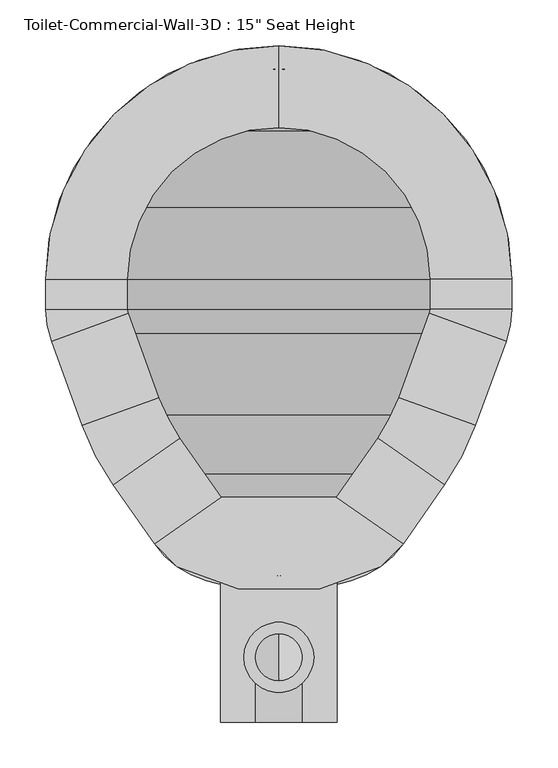
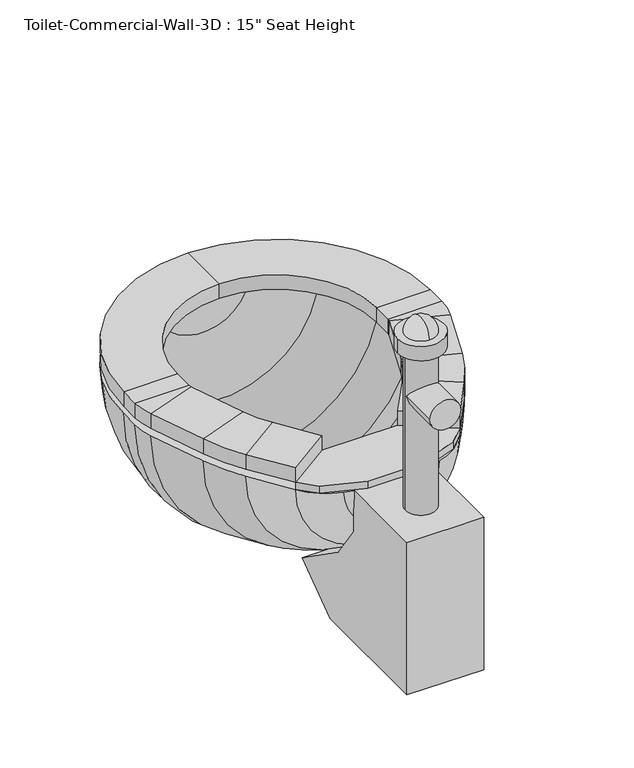
"""IFC4 building model written with IfcOpenShell, lengths in millimetres: flow terminal geometry."""

from ifc_helpers import new_model, si_unit, point, frame, frame_2d, origin, place, context, project, spatial, polyline, circle_curve, ellipse_curve, trimmed, segment, composite_curve, outline, extrude, source, transform, mapped, element, save
from ifc_brep_helpers import plane_surface, cylinder_surface, revolved_surface, advanced_brep


def flow_terminal_3100e559(model_context):
    return source(origin(), model_context, "Body", "SolidModel", [
        extrude(outline(polyline([(267.1037941, 342.9), (267.1037941, 269.296452), (310.8103185, 206.8770663), (414.8426282, 134.0328588), (334.3454017, 76.2), (114.3, 76.2), (114.3, 342.9), (267.1037941, 342.9)])), frame((341.4031538, 0.0, 0.0), z_axis=(1.0, 0.0, 0.0), x_axis=(0.0, 1.0, 0.0)), (0.0, 0.0, 1.0), 127.0),
        extrude(outline(composite_curve([segment(trimmed(circle_curve(frame_2d((404.9031538, 184.8352737)), 25.4), [point((379.5031538, 184.8352737))], [point((430.3031538, 184.8352737))], False, "CARTESIAN"), True, "CONTINUOUS"), segment(trimmed(circle_curve(frame_2d((404.9031538, 184.8352737)), 25.4), [point((430.3031538, 184.8352737))], [point((379.5031538, 184.8352737))], False, "CARTESIAN"), True, "CONTINUOUS")], self_intersect=False)), frame((0.0, 0.0, 342.9), z_axis=(0.0, 0.0, 1.0), x_axis=(1.0, 0.0, 0.0)), (0.0, 0.0, 1.0), 279.4),
        extrude(outline(composite_curve([segment(trimmed(circle_curve(frame_2d((544.2113641, 404.9031538)), 25.4), [point((544.2113641, 379.5031538))], [point((544.2113641, 430.3031538))], False, "CARTESIAN"), True, "CONTINUOUS"), segment(trimmed(circle_curve(frame_2d((544.2113641, 404.9031538)), 25.4), [point((544.2113641, 430.3031538))], [point((544.2113641, 379.5031538))], False, "CARTESIAN"), True, "CONTINUOUS")], self_intersect=False)), frame((0.0, 114.3, 0.0), z_axis=(0.0, 1.0, 0.0), x_axis=(0.0, 0.0, 1.0)), (0.0, 0.0, 1.0), 70.64375),
        extrude(outline(composite_curve([segment(trimmed(circle_curve(frame_2d((404.9031538, 184.8352737)), 38.1), [point((366.8031538, 184.8352737))], [point((443.0031538, 184.8352737))], False, "CARTESIAN"), True, "CONTINUOUS"), segment(trimmed(circle_curve(frame_2d((404.9031538, 184.8352737)), 38.1), [point((443.0031538, 184.8352737))], [point((366.8031538, 184.8352737))], False, "CARTESIAN"), True, "CONTINUOUS")], self_intersect=False)), frame((0.0, 0.0, 622.3), z_axis=(0.0, 0.0, 1.0), x_axis=(1.0, 0.0, 0.0)), (0.0, 0.0, 1.0), 25.4),
        advanced_brep(
        [(404.9031538, 159.2176912, 647.7), (404.9031538, 210.4528563, 647.7), (404.9031538, 184.8352737, 673.3175826), (404.9031538, 184.8352737, 647.7)],
        [
            (0, 1, circle_curve(frame((404.9031538, 184.8352737, 647.7), z_axis=(0.0, 0.0, 1.0), x_axis=(0.0, 1.0, 0.0)), 25.6175826)),
            (1, 2, circle_curve(frame((404.9031538, 184.8352737, 647.7), z_axis=(1.0, 0.0, 0.0), x_axis=(0.0, -1.0, 0.0)), 25.6175826)),
            (2, 0, circle_curve(frame((404.9031538, 184.8352737, 647.7), z_axis=(1.0, 0.0, 0.0), x_axis=(0.0, 1.0, 0.0)), 25.6175826)),
            (1, 0, circle_curve(frame((404.9031538, 184.8352737, 647.7), z_axis=(0.0, 0.0, 1.0), x_axis=(0.0, 1.0, 0.0)), 25.6175826)),
            (3, 1),
            (0, 3),
        ],
        [
            revolved_surface(trimmed(ellipse_curve(frame((404.9031538, 184.8352737, 647.7), z_axis=(-1.0, 0.0, 0.0), x_axis=(0.0, -1.0, 0.0)), 25.6175826, 25.6175826), [point((404.9031538, 184.8352737, 673.3175826))], [point((404.9031538, 210.4528563, 647.7))], True, "CARTESIAN"), (404.9031538, 184.8352737, 712.3277273), (0.0, 0.0, -1.0)),
            plane_surface(frame((404.9031538, 184.8352737, 647.7), z_axis=(0.0, 0.0, -1.0), x_axis=(0.0, 1.0, 0.0))),
        ],
        [
            (0, [[1, 2, 3]]),
            (0, [[4, -3, -2]]),
            (1, [[5, -1, 6]]),
            (1, [[-6, -4, -5]]),
        ],
    ),
        advanced_brep(
        [(491.7762702, 835.5819257, 342.9), (404.9031538, 850.9, 342.9), (404.9031538, 825.5, 342.9), (483.0889586, 811.7137331, 342.9), (566.547764, 758.5446102, 342.9), (619.7168869, 675.0858048, 342.9), (633.5031538, 596.9, 342.9), (633.5031538, 564.0148212, 342.9), (628.9077315, 537.9528863, 342.9), (596.6355667, 449.2858422, 342.9), (562.9565296, 384.5890139, 342.9), (525.0728964, 330.4855786, 342.9), (468.1430637, 290.6228806, 342.9), (404.9031538, 273.6777978, 342.9), (404.9031538, 247.3817829, 342.9), (483.6469009, 268.4811063, 342.9), (540.5767337, 308.3438043, 342.9), (585.6810159, 372.7593951, 342.9), (619.360053, 437.4562234, 342.9), (652.7759241, 529.2655747, 342.9), (658.9031538, 564.0148212, 342.9), (658.9031538, 596.9, 342.9), (643.5850795, 683.7731164, 342.9), (584.5082762, 776.5051224, 342.9), (318.0300374, 835.5819257, 342.9), (225.2980314, 776.5051224, 342.9), (166.2212281, 683.7731164, 342.9), (150.9031538, 596.9, 342.9), (150.9031538, 564.0148212, 342.9), (157.0303835, 529.2655747, 342.9), (190.4462546, 437.4562234, 342.9), (224.1252917, 372.7593951, 342.9), (269.229574, 308.3438043, 342.9), (326.1594067, 268.4811063, 342.9), (341.663244, 290.6228806, 342.9), (284.7334112, 330.4855786, 342.9), (246.849778, 384.5890139, 342.9), (213.1707409, 449.2858422, 342.9), (180.8985761, 537.9528863, 342.9), (176.3031538, 564.0148212, 342.9), (176.3031538, 596.9, 342.9), (190.0894207, 675.0858048, 342.9), (243.2585436, 758.5446102, 342.9), (326.7173491, 811.7137331, 342.9)],
        [
            (0, 1, circle_curve(frame((404.9031538, 596.9, 342.9), z_axis=(0.0, 0.0, 1.0), x_axis=(1.0, 0.0, 0.0)), 254.0)),
            (1, 2),
            (2, 3, circle_curve(frame((404.9031538, 596.9, 342.9), z_axis=(0.0, 0.0, -1.0), x_axis=(1.0, 0.0, 0.0)), 228.6)),
            (3, 4, circle_curve(frame((404.9031538, 596.9, 342.9), z_axis=(0.0, 0.0, -1.0), x_axis=(1.0, 0.0, 0.0)), 228.6)),
            (4, 5, circle_curve(frame((404.9031538, 596.9, 342.9), z_axis=(0.0, 0.0, -1.0), x_axis=(1.0, 0.0, 0.0)), 228.6)),
            (5, 6, circle_curve(frame((404.9031538, 596.9, 342.9), z_axis=(0.0, 0.0, -1.0), x_axis=(1.0, 0.0, 0.0)), 228.6)),
            (6, 7),
            (7, 8, circle_curve(frame((557.3031538, 564.0148212, 342.9), z_axis=(0.0, 0.0, -1.0), x_axis=(1.0, 0.0, 0.0)), 76.2)),
            (8, 9),
            (9, 10, circle_curve(frame((334.0854485, 544.8462703, 342.9), z_axis=(0.0, 0.0, -1.0), x_axis=(1.0, 0.0, 0.0)), 279.4)),
            (10, 11),
            (11, 12, circle_curve(frame((441.8470487, 388.7609446, 342.9), z_axis=(0.0, 0.0, -1.0), x_axis=(1.0, 0.0, 0.0)), 101.6)),
            (12, 13),
            (13, 14),
            (14, 15),
            (15, 16, circle_curve(frame((457.350886, 366.6191703, 342.9), z_axis=(0.0, 0.0, 1.0), x_axis=(1.0, 0.0, 0.0)), 101.6)),
            (16, 17),
            (17, 18, circle_curve(frame((356.8099347, 533.0166514, 342.9), z_axis=(0.0, 0.0, 1.0), x_axis=(1.0, 0.0, 0.0)), 279.4)),
            (18, 19),
            (19, 20, circle_curve(frame((557.3031538, 564.0148212, 342.9), z_axis=(0.0, 0.0, 1.0), x_axis=(1.0, 0.0, 0.0)), 101.6)),
            (20, 21),
            (21, 22, circle_curve(frame((404.9031538, 596.9, 342.9), z_axis=(0.0, 0.0, 1.0), x_axis=(1.0, 0.0, 0.0)), 254.0)),
            (22, 23, circle_curve(frame((404.9031538, 596.9, 342.9), z_axis=(0.0, 0.0, 1.0), x_axis=(1.0, 0.0, 0.0)), 254.0)),
            (23, 0, circle_curve(frame((404.9031538, 596.9, 342.9), z_axis=(0.0, 0.0, 1.0), x_axis=(1.0, 0.0, 0.0)), 254.0)),
            (24, 25, circle_curve(frame((404.9031538, 596.9, 342.9), z_axis=(0.0, 0.0, 1.0), x_axis=(-1.0, 0.0, 0.0)), 254.0)),
            (25, 26, circle_curve(frame((404.9031538, 596.9, 342.9), z_axis=(0.0, 0.0, 1.0), x_axis=(-1.0, 0.0, 0.0)), 254.0)),
            (26, 27, circle_curve(frame((404.9031538, 596.9, 342.9), z_axis=(0.0, 0.0, 1.0), x_axis=(-1.0, 0.0, 0.0)), 254.0)),
            (27, 28),
            (28, 29, circle_curve(frame((252.5031538, 564.0148212, 342.9), z_axis=(0.0, 0.0, 1.0), x_axis=(-1.0, 0.0, 0.0)), 101.6)),
            (29, 30),
            (30, 31, circle_curve(frame((452.9963729, 533.0166514, 342.9), z_axis=(0.0, 0.0, 1.0), x_axis=(-1.0, 0.0, 0.0)), 279.4)),
            (31, 32),
            (32, 33, circle_curve(frame((352.4554217, 366.6191703, 342.9), z_axis=(0.0, 0.0, 1.0), x_axis=(-1.0, 0.0, 0.0)), 101.6)),
            (33, 14),
            (13, 34),
            (34, 35, circle_curve(frame((367.9592589, 388.7609446, 342.9), z_axis=(0.0, 0.0, -1.0), x_axis=(-1.0, 0.0, 0.0)), 101.6)),
            (35, 36),
            (36, 37, circle_curve(frame((475.7208592, 544.8462703, 342.9), z_axis=(0.0, 0.0, -1.0), x_axis=(-1.0, 0.0, 0.0)), 279.4)),
            (37, 38),
            (38, 39, circle_curve(frame((252.5031538, 564.0148212, 342.9), z_axis=(0.0, 0.0, -1.0), x_axis=(-1.0, 0.0, 0.0)), 76.2)),
            (39, 40),
            (40, 41, circle_curve(frame((404.9031538, 596.9, 342.9), z_axis=(0.0, 0.0, -1.0), x_axis=(-1.0, 0.0, 0.0)), 228.6)),
            (41, 42, circle_curve(frame((404.9031538, 596.9, 342.9), z_axis=(0.0, 0.0, -1.0), x_axis=(-1.0, 0.0, 0.0)), 228.6)),
            (42, 43, circle_curve(frame((404.9031538, 596.9, 342.9), z_axis=(0.0, 0.0, -1.0), x_axis=(-1.0, 0.0, 0.0)), 228.6)),
            (43, 2, circle_curve(frame((404.9031538, 596.9, 342.9), z_axis=(0.0, 0.0, -1.0), x_axis=(-1.0, 0.0, 0.0)), 228.6)),
            (1, 24, circle_curve(frame((404.9031538, 596.9, 342.9), z_axis=(0.0, 0.0, 1.0), x_axis=(-1.0, 0.0, 0.0)), 254.0)),
            (0, 24, circle_curve(frame((404.9031538, 835.5819257, 342.9), z_axis=(0.0, 1.0, 0.0), x_axis=(1.0, 0.0, 0.0)), 86.8731164)),
            (43, 3, circle_curve(frame((404.9031538, 811.7137331, 342.9), z_axis=(0.0, -1.0, 0.0), x_axis=(1.0, 0.0, 0.0)), 78.1858048)),
            (42, 4, circle_curve(frame((404.9031538, 758.5446102, 342.9), z_axis=(0.0, -1.0, 0.0), x_axis=(1.0, 0.0, 0.0)), 161.6446102)),
            (41, 5, circle_curve(frame((404.9031538, 675.0858048, 342.9), z_axis=(0.0, -1.0, 0.0), x_axis=(1.0, 0.0, 0.0)), 214.8137331)),
            (40, 6, circle_curve(frame((404.9031538, 596.9, 342.9), z_axis=(0.0, -1.0, 0.0), x_axis=(1.0, 0.0, 0.0)), 228.6)),
            (39, 7, circle_curve(frame((404.9031538, 564.0148212, 342.9), z_axis=(0.0, -1.0, 0.0), x_axis=(1.0, 0.0, 0.0)), 228.6)),
            (38, 8, circle_curve(frame((404.9031538, 537.9528863, 342.9), z_axis=(0.0, -1.0, 0.0), x_axis=(1.0, 0.0, 0.0)), 224.0045777)),
            (37, 9, circle_curve(frame((404.9031538, 449.2858422, 342.9), z_axis=(0.0, -1.0, 0.0), x_axis=(1.0, 0.0, 0.0)), 191.7324129)),
            (36, 10, circle_curve(frame((404.9031538, 384.5890139, 342.9), z_axis=(0.0, -1.0, 0.0), x_axis=(1.0, 0.0, 0.0)), 158.0533758)),
            (35, 11, circle_curve(frame((404.9031538, 330.4855786, 342.9), z_axis=(0.0, -1.0, 0.0), x_axis=(1.0, 0.0, 0.0)), 120.1697426)),
            (34, 12, circle_curve(frame((404.9031538, 290.6228806, 342.9), z_axis=(0.0, -1.0, 0.0), x_axis=(1.0, 0.0, 0.0)), 63.2399099)),
            (33, 15, circle_curve(frame((404.9031538, 268.4811063, 342.9), z_axis=(0.0, -1.0, 0.0), x_axis=(1.0, 0.0, 0.0)), 78.7437471)),
            (32, 16, circle_curve(frame((404.9031538, 308.3438043, 342.9), z_axis=(0.0, -1.0, 0.0), x_axis=(1.0, 0.0, 0.0)), 135.6735798)),
            (31, 17, circle_curve(frame((404.9031538, 372.7593951, 342.9), z_axis=(0.0, -1.0, 0.0), x_axis=(1.0, 0.0, 0.0)), 180.7778621)),
            (30, 18, circle_curve(frame((404.9031538, 437.4562234, 342.9), z_axis=(0.0, -1.0, 0.0), x_axis=(1.0, 0.0, 0.0)), 214.4568992)),
            (29, 19, circle_curve(frame((404.9031538, 529.2655747, 342.9), z_axis=(0.0, -1.0, 0.0), x_axis=(1.0, 0.0, 0.0)), 247.8727703)),
            (28, 20, circle_curve(frame((404.9031538, 564.0148212, 342.9), z_axis=(0.0, -1.0, 0.0), x_axis=(1.0, 0.0, 0.0)), 254.0)),
            (27, 21, circle_curve(frame((404.9031538, 596.9, 342.9), z_axis=(0.0, -1.0, 0.0), x_axis=(1.0, 0.0, 0.0)), 254.0)),
            (26, 22, circle_curve(frame((404.9031538, 683.7731164, 342.9), z_axis=(0.0, -1.0, 0.0), x_axis=(1.0, 0.0, 0.0)), 238.6819257)),
            (25, 23, circle_curve(frame((404.9031538, 776.5051224, 342.9), z_axis=(0.0, -1.0, 0.0), x_axis=(1.0, 0.0, 0.0)), 179.6051224)),
        ],
        [
            plane_surface(frame((404.9031538, 956.1102448, 342.9), z_axis=(0.0, 0.0, 1.0), x_axis=(1.0, 0.0, 0.0))),
            plane_surface(frame((404.9031538, 956.1102448, 342.9), z_axis=(0.0, 0.0, 1.0), x_axis=(-1.0, 0.0, 0.0))),
            revolved_surface(trimmed(ellipse_curve(frame((404.9031538, 596.9, 342.9), z_axis=(0.0, 0.0, 1.0), x_axis=(1.0, 0.0, 0.0)), 254.0, 254.0), [point((491.7762702, 835.5819257, 342.9))], [point((404.9031538, 850.9, 342.9))], True, "CARTESIAN"), (404.9031538, 956.1102448, 342.9), (0.0, 1.0, 0.0)),
            revolved_surface(trimmed(ellipse_curve(frame((404.9031538, 596.9, 342.9), z_axis=(0.0, 0.0, -1.0), x_axis=(1.0, 0.0, 0.0)), 228.6, 228.6), [point((404.9031538, 825.5, 342.9))], [point((483.0889586, 811.7137331, 342.9))], True, "CARTESIAN"), (404.9031538, 956.1102448, 342.9), (0.0, 1.0, 0.0)),
            revolved_surface(trimmed(ellipse_curve(frame((404.9031538, 596.9, 342.9), z_axis=(0.0, 0.0, -1.0), x_axis=(1.0, 0.0, 0.0)), 228.6, 228.6), [point((483.0889586, 811.7137331, 342.9))], [point((566.547764, 758.5446102, 342.9))], True, "CARTESIAN"), (404.9031538, 956.1102448, 342.9), (0.0, 1.0, 0.0)),
            revolved_surface(trimmed(ellipse_curve(frame((404.9031538, 596.9, 342.9), z_axis=(0.0, 0.0, -1.0), x_axis=(1.0, 0.0, 0.0)), 228.6, 228.6), [point((566.547764, 758.5446102, 342.9))], [point((619.7168869, 675.0858048, 342.9))], True, "CARTESIAN"), (404.9031538, 956.1102448, 342.9), (0.0, 1.0, 0.0)),
            revolved_surface(trimmed(ellipse_curve(frame((404.9031538, 596.9, 342.9), z_axis=(0.0, 0.0, -1.0), x_axis=(1.0, 0.0, 0.0)), 228.6, 228.6), [point((619.7168869, 675.0858048, 342.9))], [point((633.5031538, 596.9, 342.9))], True, "CARTESIAN"), (404.9031538, 956.1102448, 342.9), (0.0, 1.0, 0.0)),
            revolved_surface(polyline([(633.5031538, 596.9, 342.9), (633.5031538, 564.0148212, 342.9)]), (404.9031538, 956.1102448, 342.9), (0.0, 1.0, 0.0)),
            revolved_surface(trimmed(ellipse_curve(frame((557.3031538, 564.0148212, 342.9), z_axis=(0.0, 0.0, -1.0), x_axis=(1.0, 0.0, 0.0)), 76.2, 76.2), [point((633.5031538, 564.0148212, 342.9))], [point((628.9077315, 537.9528863, 342.9))], True, "CARTESIAN"), (404.9031538, 956.1102448, 342.9), (0.0, 1.0, 0.0)),
            revolved_surface(polyline([(628.9077315, 537.9528863, 342.9), (596.6355667, 449.2858422, 342.9)]), (404.9031538, 956.1102448, 342.9), (0.0, 1.0, 0.0)),
            revolved_surface(trimmed(ellipse_curve(frame((334.0854485, 544.8462703, 342.9), z_axis=(0.0, 0.0, -1.0), x_axis=(1.0, 0.0, 0.0)), 279.4, 279.4), [point((596.6355667, 449.2858422, 342.9))], [point((562.9565296, 384.5890139, 342.9))], True, "CARTESIAN"), (404.9031538, 956.1102448, 342.9), (0.0, 1.0, 0.0)),
            revolved_surface(polyline([(562.9565296, 384.5890139, 342.9), (525.0728964, 330.4855786, 342.9)]), (404.9031538, 956.1102448, 342.9), (0.0, 1.0, 0.0)),
            revolved_surface(trimmed(ellipse_curve(frame((441.8470487, 388.7609446, 342.9), z_axis=(0.0, 0.0, -1.0), x_axis=(1.0, 0.0, 0.0)), 101.6, 101.6), [point((525.0728964, 330.4855786, 342.9))], [point((468.1430637, 290.6228806, 342.9))], True, "CARTESIAN"), (404.9031538, 956.1102448, 342.9), (0.0, 1.0, 0.0)),
            revolved_surface(polyline([(468.1430637, 290.6228806, 342.9), (404.9031538, 273.6777978, 342.9)]), (404.9031538, 956.1102448, 342.9), (0.0, 1.0, 0.0)),
            revolved_surface(polyline([(404.9031538, 247.3817829, 342.9), (483.6469009, 268.4811063, 342.9)]), (404.9031538, 956.1102448, 342.9), (0.0, 1.0, 0.0)),
            revolved_surface(trimmed(ellipse_curve(frame((457.350886, 366.6191703, 342.9), z_axis=(0.0, 0.0, 1.0), x_axis=(1.0, 0.0, 0.0)), 101.6, 101.6), [point((483.6469009, 268.4811063, 342.9))], [point((540.5767337, 308.3438043, 342.9))], True, "CARTESIAN"), (404.9031538, 956.1102448, 342.9), (0.0, 1.0, 0.0)),
            revolved_surface(polyline([(540.5767337, 308.3438043, 342.9), (585.6810159, 372.7593951, 342.9)]), (404.9031538, 956.1102448, 342.9), (0.0, 1.0, 0.0)),
            revolved_surface(trimmed(ellipse_curve(frame((356.8099347, 533.0166514, 342.9), z_axis=(0.0, 0.0, 1.0), x_axis=(1.0, 0.0, 0.0)), 279.4, 279.4), [point((585.6810159, 372.7593951, 342.9))], [point((619.360053, 437.4562234, 342.9))], True, "CARTESIAN"), (404.9031538, 956.1102448, 342.9), (0.0, 1.0, 0.0)),
            revolved_surface(polyline([(619.360053, 437.4562234, 342.9), (652.7759241, 529.2655747, 342.9)]), (404.9031538, 956.1102448, 342.9), (0.0, 1.0, 0.0)),
            revolved_surface(trimmed(ellipse_curve(frame((557.3031538, 564.0148212, 342.9), z_axis=(0.0, 0.0, 1.0), x_axis=(1.0, 0.0, 0.0)), 101.6, 101.6), [point((652.7759241, 529.2655747, 342.9))], [point((658.9031538, 564.0148212, 342.9))], True, "CARTESIAN"), (404.9031538, 956.1102448, 342.9), (0.0, 1.0, 0.0)),
            cylinder_surface(frame((404.9031538, 956.1102448, 342.9), z_axis=(0.0, 1.0, 0.0), x_axis=(1.0, 0.0, 0.0)), 254.0),
            revolved_surface(trimmed(ellipse_curve(frame((404.9031538, 596.9, 342.9), z_axis=(0.0, 0.0, 1.0), x_axis=(1.0, 0.0, 0.0)), 254.0, 254.0), [point((658.9031538, 596.9, 342.9))], [point((643.5850795, 683.7731164, 342.9))], True, "CARTESIAN"), (404.9031538, 956.1102448, 342.9), (0.0, 1.0, 0.0)),
            revolved_surface(trimmed(ellipse_curve(frame((404.9031538, 596.9, 342.9), z_axis=(0.0, 0.0, 1.0), x_axis=(1.0, 0.0, 0.0)), 254.0, 254.0), [point((643.5850795, 683.7731164, 342.9))], [point((584.5082762, 776.5051224, 342.9))], True, "CARTESIAN"), (404.9031538, 956.1102448, 342.9), (0.0, 1.0, 0.0)),
            revolved_surface(trimmed(ellipse_curve(frame((404.9031538, 596.9, 342.9), z_axis=(0.0, 0.0, 1.0), x_axis=(1.0, 0.0, 0.0)), 254.0, 254.0), [point((584.5082762, 776.5051224, 342.9))], [point((491.7762702, 835.5819257, 342.9))], True, "CARTESIAN"), (404.9031538, 956.1102448, 342.9), (0.0, 1.0, 0.0)),
        ],
        [
            (0, [[1, 2, 3, 4, 5, 6, 7, 8, 9, 10, 11, 12, 13, 14, 15, 16, 17, 18, 19, 20, 21, 22, 23, 24]]),
            (1, [[25, 26, 27, 28, 29, 30, 31, 32, 33, 34, -14, 35, 36, 37, 38, 39, 40, 41, 42, 43, 44, 45, -2, 46]]),
            (2, [[-1, 47, -46]]),
            (3, [[48, -3, -45]]),
            (4, [[49, -4, -48, -44]]),
            (5, [[50, -5, -49, -43]]),
            (6, [[51, -6, -50, -42]]),
            (7, [[52, -7, -51, -41]]),
            (8, [[53, -8, -52, -40]]),
            (9, [[54, -9, -53, -39]]),
            (10, [[55, -10, -54, -38]]),
            (11, [[56, -11, -55, -37]]),
            (12, [[57, -12, -56, -36]]),
            (13, [[-13, -57, -35]]),
            (14, [[58, -15, -34]]),
            (15, [[59, -16, -58, -33]]),
            (16, [[60, -17, -59, -32]]),
            (17, [[61, -18, -60, -31]]),
            (18, [[62, -19, -61, -30]]),
            (19, [[63, -20, -62, -29]]),
            (20, [[64, -21, -63, -28]]),
            (21, [[65, -22, -64, -27]]),
            (22, [[66, -23, -65, -26]]),
            (23, [[-47, -24, -66, -25]]),
        ],
    ),
        advanced_brep(
        [(467.7541169, 359.3347495, 355.6), (540.5767337, 308.3438043, 355.6), (540.5767337, 308.3438043, 381.0), (467.7541169, 359.3347495, 381.0), (512.8583992, 423.7503403, 355.6), (585.6810159, 372.7593951, 355.6), (585.6810159, 372.7593951, 381.0), (512.8583992, 423.7503403, 381.0), (619.360053, 437.4562234, 355.6), (535.821379, 467.8618141, 355.6), (619.360053, 437.4562234, 381.0), (535.821379, 467.8618141, 381.0), (569.2372501, 559.6711654, 355.6), (652.7759241, 529.2655747, 355.6), (652.7759241, 529.2655747, 381.0), (569.2372501, 559.6711654, 381.0), (658.9031538, 564.0148212, 355.6), (570.0031538, 564.0148212, 355.6), (658.9031538, 564.0148212, 381.0), (570.0031538, 564.0148212, 381.0), (570.0031538, 596.9, 355.6), (658.9031538, 596.9, 355.6), (658.9031538, 596.9, 381.0), (570.0031538, 596.9, 381.0), (404.9031538, 850.9, 355.6), (404.9031538, 762.0, 355.6), (404.9031538, 850.9, 381.0), (404.9031538, 762.0, 381.0), (150.9031538, 596.9, 355.6), (239.8031538, 596.9, 355.6), (150.9031538, 596.9, 381.0), (239.8031538, 596.9, 381.0), (239.8031538, 564.0148212, 355.6), (150.9031538, 564.0148212, 355.6), (150.9031538, 564.0148212, 381.0), (239.8031538, 564.0148212, 381.0), (157.0303835, 529.2655747, 355.6), (240.5690575, 559.6711654, 355.6), (157.0303835, 529.2655747, 381.0), (240.5690575, 559.6711654, 381.0), (273.9849286, 467.8618141, 355.6), (190.4462546, 437.4562234, 355.6), (190.4462546, 437.4562234, 381.0), (273.9849286, 467.8618141, 381.0), (224.1252917, 372.7593951, 355.6), (296.9479084, 423.7503403, 355.6), (224.1252917, 372.7593951, 381.0), (296.9479084, 423.7503403, 381.0), (342.0521907, 359.3347495, 355.6), (342.0521907, 359.3347495, 381.0), (269.229574, 308.3438043, 381.0), (269.229574, 308.3438043, 355.6)],
        [
            (0, 1),
            (1, 2),
            (2, 3),
            (3, 0),
            (0, 4),
            (4, 5),
            (5, 1),
            (5, 6),
            (6, 2),
            (6, 7),
            (7, 3),
            (7, 4),
            (8, 5, circle_curve(frame((356.8099347, 533.0166514, 355.6), z_axis=(0.0, 0.0, -1.0), x_axis=(0.81915204428899, -0.5735764363510486, 0.0)), 279.4)),
            (4, 9, circle_curve(frame((356.8099347, 533.0166514, 355.6), z_axis=(0.0, 0.0, 1.0), x_axis=(0.81915204428899, -0.5735764363510486, 0.0)), 190.5)),
            (9, 8),
            (10, 6, circle_curve(frame((356.8099347, 533.0166514, 381.0), z_axis=(0.0, 0.0, -1.0), x_axis=(0.81915204428899, -0.5735764363510486, 0.0)), 279.4)),
            (8, 10),
            (11, 7, circle_curve(frame((356.8099347, 533.0166514, 381.0), z_axis=(0.0, 0.0, -1.0), x_axis=(0.81915204428899, -0.5735764363510486, 0.0)), 190.5)),
            (10, 11),
            (11, 9),
            (9, 12),
            (12, 13),
            (13, 8),
            (13, 14),
            (14, 10),
            (14, 15),
            (15, 11),
            (15, 12),
            (16, 13, circle_curve(frame((557.3031538, 564.0148212, 355.6), z_axis=(0.0, 0.0, -1.0), x_axis=(0.939692620785906, -0.34202014332567526, 0.0)), 101.6)),
            (12, 17, circle_curve(frame((557.3031538, 564.0148212, 355.6), z_axis=(0.0, 0.0, 1.0), x_axis=(0.939692620785906, -0.34202014332567526, 0.0)), 12.7)),
            (17, 16),
            (18, 14, circle_curve(frame((557.3031538, 564.0148212, 381.0), z_axis=(0.0, 0.0, -1.0), x_axis=(0.939692620785906, -0.34202014332567526, 0.0)), 101.6)),
            (16, 18),
            (19, 15, circle_curve(frame((557.3031538, 564.0148212, 381.0), z_axis=(0.0, 0.0, -1.0), x_axis=(0.939692620785906, -0.34202014332567526, 0.0)), 12.7)),
            (18, 19),
            (19, 17),
            (17, 20),
            (20, 21),
            (21, 16),
            (21, 22),
            (22, 18),
            (22, 23),
            (23, 19),
            (23, 20),
            (24, 21, circle_curve(frame((404.9031538, 596.9, 355.6), z_axis=(0.0, 0.0, -1.0), x_axis=(1.0, 0.0, 0.0)), 254.0)),
            (20, 25, circle_curve(frame((404.9031538, 596.9, 355.6), z_axis=(0.0, 0.0, 1.0), x_axis=(1.0, 0.0, 0.0)), 165.1)),
            (25, 24),
            (26, 22, circle_curve(frame((404.9031538, 596.9, 381.0), z_axis=(0.0, 0.0, -1.0), x_axis=(1.0, 0.0, 0.0)), 254.0)),
            (24, 26),
            (27, 23, circle_curve(frame((404.9031538, 596.9, 381.0), z_axis=(0.0, 0.0, -1.0), x_axis=(1.0, 0.0, 0.0)), 165.1)),
            (26, 27),
            (27, 25),
            (28, 24, circle_curve(frame((404.9031538, 596.9, 355.6), z_axis=(0.0, 0.0, -1.0), x_axis=(0.0, 1.0, 0.0)), 254.0)),
            (25, 29, circle_curve(frame((404.9031538, 596.9, 355.6), z_axis=(0.0, 0.0, 1.0), x_axis=(0.0, 1.0, 0.0)), 165.1)),
            (29, 28),
            (30, 26, circle_curve(frame((404.9031538, 596.9, 381.0), z_axis=(0.0, 0.0, -1.0), x_axis=(0.0, 1.0, 0.0)), 254.0)),
            (28, 30),
            (31, 27, circle_curve(frame((404.9031538, 596.9, 381.0), z_axis=(0.0, 0.0, -1.0), x_axis=(0.0, 1.0, 0.0)), 165.1)),
            (30, 31),
            (31, 29),
            (29, 32),
            (32, 33),
            (33, 28),
            (33, 34),
            (34, 30),
            (34, 35),
            (35, 31),
            (35, 32),
            (36, 33, circle_curve(frame((252.5031538, 564.0148212, 355.6), z_axis=(0.0, 0.0, -1.0), x_axis=(-1.0, 0.0, 0.0)), 101.6)),
            (32, 37, circle_curve(frame((252.5031538, 564.0148212, 355.6), z_axis=(0.0, 0.0, 1.0), x_axis=(-1.0, 0.0, 0.0)), 12.7)),
            (37, 36),
            (38, 34, circle_curve(frame((252.5031538, 564.0148212, 381.0), z_axis=(0.0, 0.0, -1.0), x_axis=(-1.0, 0.0, 0.0)), 101.6)),
            (36, 38),
            (39, 35, circle_curve(frame((252.5031538, 564.0148212, 381.0), z_axis=(0.0, 0.0, -1.0), x_axis=(-1.0, 0.0, 0.0)), 12.7)),
            (38, 39),
            (39, 37),
            (37, 40),
            (40, 41),
            (41, 36),
            (41, 42),
            (42, 38),
            (42, 43),
            (43, 39),
            (43, 40),
            (44, 41, circle_curve(frame((452.9963729, 533.0166514, 355.6), z_axis=(0.0, 0.0, -1.0), x_axis=(-0.9396926207859088, -0.34202014332566766, 0.0)), 279.4)),
            (40, 45, circle_curve(frame((452.9963729, 533.0166514, 355.6), z_axis=(0.0, 0.0, 1.0), x_axis=(-0.9396926207859088, -0.34202014332566766, 0.0)), 190.5)),
            (45, 44),
            (46, 42, circle_curve(frame((452.9963729, 533.0166514, 381.0), z_axis=(0.0, 0.0, -1.0), x_axis=(-0.9396926207859088, -0.34202014332566766, 0.0)), 279.4)),
            (44, 46),
            (47, 43, circle_curve(frame((452.9963729, 533.0166514, 381.0), z_axis=(0.0, 0.0, -1.0), x_axis=(-0.9396926207859088, -0.34202014332566766, 0.0)), 190.5)),
            (46, 47),
            (47, 45),
            (48, 49),
            (49, 50),
            (50, 51),
            (51, 48),
            (45, 48),
            (51, 44),
            (50, 46),
            (49, 47),
        ],
        [
            plane_surface(frame((540.5767337, 308.3438043, 439.6203184), z_axis=(-0.5735764363510383, -0.8191520442889972, 0.0), x_axis=(0.8191520442889972, -0.5735764363510383, 0.0))),
            plane_surface(frame((467.7541169, 359.3347495, 355.6), z_axis=(0.0, 0.0, -1.0), x_axis=(0.5735764363510379, 0.8191520442889975, 0.0))),
            plane_surface(frame((540.5767337, 308.3438043, 355.6), z_axis=(0.8191520442889973, -0.5735764363510382, 0.0), x_axis=(0.5735764363510382, 0.8191520442889973, 0.0))),
            plane_surface(frame((540.5767337, 308.3438043, 381.0), z_axis=(0.0, 0.0, 1.0), x_axis=(0.5735764363510382, 0.8191520442889973, 0.0))),
            plane_surface(frame((467.7541169, 359.3347495, 381.0), z_axis=(-0.8191520442889971, 0.5735764363510386, 0.0), x_axis=(0.5735764363510386, 0.8191520442889971, 0.0))),
            plane_surface(frame((356.8099347, 533.0166514, 355.6), z_axis=(0.0, 0.0, -1.0), x_axis=(0.81915204428899, -0.5735764363510486, 0.0))),
            cylinder_surface(frame((356.8099347, 533.0166514, 342.9), z_axis=(0.0, 0.0, 1.0), x_axis=(0.81915204428899, -0.5735764363510486, 0.0)), 279.4),
            plane_surface(frame((356.8099347, 533.0166514, 381.0), z_axis=(0.0, 0.0, 1.0), x_axis=(0.81915204428899, -0.5735764363510486, 0.0))),
            revolved_surface(polyline([(512.8583991370526, 423.75034027512527, 381.0), (512.8583991370526, 423.75034027512527, 355.6)]), (356.8099347, 533.0166514, 342.9), (0.0, 0.0, 1.0)),
            plane_surface(frame((535.821379, 467.8618141, 355.6), z_axis=(0.0, 0.0, -1.0), x_axis=(0.34202014332566494, 0.9396926207859098, 0.0))),
            plane_surface(frame((619.360053, 437.4562234, 355.6), z_axis=(0.93969262078591, -0.34202014332566427, 0.0), x_axis=(0.34202014332566427, 0.93969262078591, 0.0))),
            plane_surface(frame((619.360053, 437.4562234, 381.0), z_axis=(0.0, 0.0, 1.0), x_axis=(0.34202014332566427, 0.93969262078591, 0.0))),
            plane_surface(frame((535.821379, 467.8618141, 381.0), z_axis=(-0.9396926207859095, 0.34202014332566555, 0.0), x_axis=(0.34202014332566555, 0.9396926207859095, 0.0))),
            plane_surface(frame((557.3031538, 564.0148212, 355.6), z_axis=(0.0, 0.0, -1.0), x_axis=(0.939692620785906, -0.34202014332567526, 0.0))),
            cylinder_surface(frame((557.3031538, 564.0148212, 342.9), z_axis=(0.0, 0.0, 1.0), x_axis=(0.939692620785906, -0.34202014332567526, 0.0)), 101.6),
            plane_surface(frame((557.3031538, 564.0148212, 381.0), z_axis=(0.0, 0.0, 1.0), x_axis=(0.939692620785906, -0.34202014332567526, 0.0))),
            revolved_surface(polyline([(569.237250083981, 559.6711653797639, 381.0), (569.237250083981, 559.6711653797639, 355.6)]), (557.3031538, 564.0148212, 342.9), (0.0, 0.0, 1.0)),
            plane_surface(frame((570.0031538, 564.0148212, 355.6), z_axis=(0.0, 0.0, -1.0), x_axis=(0.0, 1.0, 0.0))),
            plane_surface(frame((658.9031538, 564.0148212, 355.6), z_axis=(1.0, 0.0, 0.0), x_axis=(0.0, 1.0, 0.0))),
            plane_surface(frame((658.9031538, 564.0148212, 381.0), z_axis=(0.0, 0.0, 1.0), x_axis=(0.0, 1.0, 0.0))),
            plane_surface(frame((570.0031538, 564.0148212, 381.0), z_axis=(-1.0, 0.0, 0.0), x_axis=(0.0, 1.0, 0.0))),
            plane_surface(frame((404.9031538, 596.9, 355.6), z_axis=(0.0, 0.0, -1.0), x_axis=(1.0, 0.0, 0.0))),
            cylinder_surface(frame((404.9031538, 596.9, 342.9), z_axis=(0.0, 0.0, 1.0), x_axis=(1.0, 0.0, 0.0)), 254.0),
            plane_surface(frame((404.9031538, 596.9, 381.0), z_axis=(0.0, 0.0, 1.0), x_axis=(1.0, 0.0, 0.0))),
            revolved_surface(polyline([(570.0031538, 596.9, 381.0), (570.0031538, 596.9, 355.6)]), (404.9031538, 596.9, 342.9), (0.0, 0.0, 1.0)),
            plane_surface(frame((404.9031538, 596.9, 355.6), z_axis=(0.0, 0.0, -1.0), x_axis=(0.0, 1.0, 0.0))),
            cylinder_surface(frame((404.9031538, 596.9, 342.9), z_axis=(0.0, 0.0, 1.0), x_axis=(0.0, 1.0, 0.0)), 254.0),
            plane_surface(frame((404.9031538, 596.9, 381.0), z_axis=(0.0, 0.0, 1.0), x_axis=(0.0, 1.0, 0.0))),
            revolved_surface(polyline([(404.9031538, 762.0, 381.0), (404.9031538, 762.0, 355.6)]), (404.9031538, 596.9, 342.9), (0.0, 0.0, 1.0)),
            plane_surface(frame((239.8031538, 596.9, 355.6), z_axis=(0.0, 0.0, -1.0), x_axis=(0.0, -1.0, 0.0))),
            plane_surface(frame((150.9031538, 596.9, 355.6), z_axis=(-1.0, 0.0, 0.0), x_axis=(0.0, -1.0, 0.0))),
            plane_surface(frame((150.9031538, 596.9, 381.0), z_axis=(0.0, 0.0, 1.0), x_axis=(0.0, -1.0, 0.0))),
            plane_surface(frame((239.8031538, 596.9, 381.0), z_axis=(1.0, 0.0, 0.0), x_axis=(0.0, -1.0, 0.0))),
            plane_surface(frame((252.5031538, 564.0148212, 355.6), z_axis=(0.0, 0.0, -1.0), x_axis=(-1.0, 0.0, 0.0))),
            cylinder_surface(frame((252.5031538, 564.0148212, 342.9), z_axis=(0.0, 0.0, 1.0), x_axis=(-1.0, 0.0, 0.0)), 101.6),
            plane_surface(frame((252.5031538, 564.0148212, 381.0), z_axis=(0.0, 0.0, 1.0), x_axis=(-1.0, 0.0, 0.0))),
            revolved_surface(polyline([(239.80315380000002, 564.0148212, 381.0), (239.80315380000002, 564.0148212, 355.6)]), (252.5031538, 564.0148212, 342.9), (0.0, 0.0, 1.0)),
            plane_surface(frame((240.5690575, 559.6711654, 355.6), z_axis=(0.0, 0.0, -1.0), x_axis=(0.34202014332565583, -0.9396926207859131, 0.0))),
            plane_surface(frame((157.0303835, 529.2655747, 355.6), z_axis=(-0.9396926207859131, -0.34202014332565583, 0.0), x_axis=(0.34202014332565583, -0.9396926207859131, 0.0))),
            plane_surface(frame((157.0303835, 529.2655747, 381.0), z_axis=(0.0, 0.0, 1.0), x_axis=(0.3420201433256553, -0.9396926207859133, 0.0))),
            plane_surface(frame((240.5690575, 559.6711654, 381.0), z_axis=(0.9396926207859132, 0.3420201433256555, 0.0), x_axis=(0.3420201433256555, -0.9396926207859132, 0.0))),
            plane_surface(frame((452.9963729, 533.0166514, 355.6), z_axis=(0.0, 0.0, -1.0), x_axis=(-0.9396926207859088, -0.34202014332566766, 0.0))),
            cylinder_surface(frame((452.9963729, 533.0166514, 342.9), z_axis=(0.0, 0.0, 1.0), x_axis=(-0.9396926207859088, -0.34202014332566766, 0.0)), 279.4),
            plane_surface(frame((452.9963729, 533.0166514, 381.0), z_axis=(0.0, 0.0, 1.0), x_axis=(-0.9396926207859088, -0.34202014332566766, 0.0))),
            revolved_surface(polyline([(273.98492864028435, 467.8618140964603, 381.0), (273.98492864028435, 467.8618140964603, 355.6)]), (452.9963729, 533.0166514, 342.9), (0.0, 0.0, 1.0)),
            plane_surface(frame((269.229574, 308.3438043, 246.1796816), z_axis=(0.5735764363510503, -0.8191520442889889, 0.0), x_axis=(0.8191520442889889, 0.5735764363510503, 0.0))),
            plane_surface(frame((296.9479084, 423.7503403, 355.6), z_axis=(0.0, 0.0, -1.0000000000000002), x_axis=(0.5735764363510502, -0.819152044288989, 0.0))),
            plane_surface(frame((224.1252917, 372.7593951, 355.6), z_axis=(-0.8191520442889888, -0.5735764363510505, 0.0), x_axis=(0.5735764363510505, -0.8191520442889888, 0.0))),
            plane_surface(frame((224.1252917, 372.7593951, 381.0), z_axis=(0.0, 0.0, 1.0), x_axis=(0.5735764363510505, -0.8191520442889888, 0.0))),
            plane_surface(frame((296.9479084, 423.7503403, 381.0), z_axis=(0.8191520442889894, 0.5735764363510497, 0.0), x_axis=(0.5735764363510497, -0.8191520442889894, 0.0))),
        ],
        [
            (0, [[1, 2, 3, 4]]),
            (1, [[-1, 5, 6, 7]]),
            (2, [[-2, -7, 8, 9]]),
            (3, [[-3, -9, 10, 11]]),
            (4, [[-4, -11, 12, -5]]),
            (5, [[13, -6, 14, 15]]),
            (6, [[16, -8, -13, 17]]),
            (7, [[18, -10, -16, 19]]),
            (8, [[-14, -12, -18, 20]]),
            (9, [[-15, 21, 22, 23]]),
            (10, [[-17, -23, 24, 25]]),
            (11, [[-19, -25, 26, 27]]),
            (12, [[-20, -27, 28, -21]]),
            (13, [[29, -22, 30, 31]]),
            (14, [[32, -24, -29, 33]]),
            (15, [[34, -26, -32, 35]]),
            (16, [[-30, -28, -34, 36]]),
            (17, [[-31, 37, 38, 39]]),
            (18, [[-33, -39, 40, 41]]),
            (19, [[-35, -41, 42, 43]]),
            (20, [[-36, -43, 44, -37]]),
            (21, [[45, -38, 46, 47]]),
            (22, [[48, -40, -45, 49]]),
            (23, [[50, -42, -48, 51]]),
            (24, [[-46, -44, -50, 52]]),
            (25, [[53, -47, 54, 55]]),
            (26, [[56, -49, -53, 57]]),
            (27, [[58, -51, -56, 59]]),
            (28, [[-54, -52, -58, 60]]),
            (29, [[-55, 61, 62, 63]]),
            (30, [[-57, -63, 64, 65]]),
            (31, [[-59, -65, 66, 67]]),
            (32, [[-60, -67, 68, -61]]),
            (33, [[69, -62, 70, 71]]),
            (34, [[72, -64, -69, 73]]),
            (35, [[74, -66, -72, 75]]),
            (36, [[-70, -68, -74, 76]]),
            (37, [[-71, 77, 78, 79]]),
            (38, [[-73, -79, 80, 81]]),
            (39, [[-75, -81, 82, 83]]),
            (40, [[-76, -83, 84, -77]]),
            (41, [[85, -78, 86, 87]]),
            (42, [[88, -80, -85, 89]]),
            (43, [[90, -82, -88, 91]]),
            (44, [[-86, -84, -90, 92]]),
            (45, [[93, 94, 95, 96]]),
            (46, [[-87, 97, -96, 98]]),
            (47, [[-89, -98, -95, 99]]),
            (48, [[-91, -99, -94, 100]]),
            (49, [[-92, -100, -93, -97]]),
        ],
    ),
        extrude(outline(polyline([(467.7541169, 359.3347495), (540.5767337, 308.3438043), (515.6262519, 283.3933226), (449.563909, 259.3485961), (360.2423986, 259.3485961), (294.1800557, 283.3933226), (269.229574, 308.3438043), (342.0521907, 359.3347495), (467.7541169, 359.3347495)])), frame((0.0, 0.0, 342.9), z_axis=(0.0, 0.0, 1.0), x_axis=(1.0, 0.0, 0.0)), (0.0, 0.0, 1.0), 12.7),
    ])


if __name__ == "__main__":
    model = new_model("IFC4")
    model_context = context("Model", 3, world=origin())
    ifc_project = project(units=[si_unit("LENGTHUNIT", "METRE", prefix="MILLI")], contexts=[model_context])
    site = spatial("IfcSite", under=ifc_project)
    building = spatial("IfcBuilding", under=site)
    placement = place(None, origin())
    flow_terminal_shape = flow_terminal_3100e559(model_context)
    element("IfcFlowTerminal", 1, ObjectType="Toilet-Commercial-Wall-3D : 15\" Seat Height", at=placement, inside=building, context=model_context, shape_type="MappedRepresentation", body=[
        mapped(flow_terminal_shape, transform((0.0, 0.0, 0.0), x_axis=(1.0, 0.0, 0.0), y_axis=(0.0, 1.0, 0.0), z_axis=(0.0, 0.0, 1.0))),
    ])
    save(model, "model.ifc")

# Revit data of these elements
# Type "Toilet-Commercial-Wall-3D : 15\" Seat Height"
#   Assembly Code = "D2010110"
#   Mounting Height = 1' - 3"
#   Piping Material = Steel, Polished
#   Toilet - Bowl Material = Porcelain, Ivory
#   Toilet - Seat Material = Laminate, Ivory, Matte
#   Default Elevation = 0
# Element 1 (IfcFlowTerminal, "Toilet-Commercial-Wall-3D : 15\" Seat Height")
#   Materials on its faces: "Laminate, Ivory, Matte", "Porcelain, Ivory", "Steel, Polished"
# Materials
#   "Steel, Polished": class "Metal", colour RGB 57 57 57, transparency 0, Description = "Polished steel", Cost = 0
#   "Porcelain, Ivory": class "Ceramic", colour RGB 247 247 239, transparency 0, Description = "Porcelain, ivory", Cost = 0
#   "Laminate, Ivory, Matte": class "Plastic", colour RGB 247 247 239, transparency 0, Description = "Plastic Laminate - Ivory, Matte", Cost = 0
